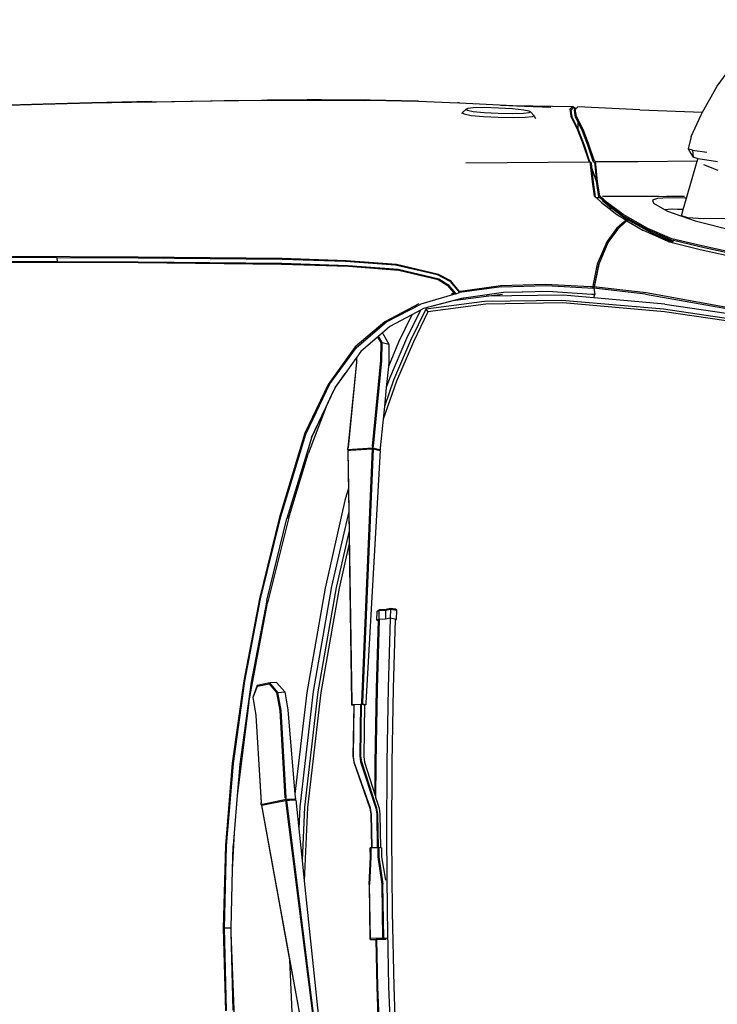
# Model space of a CAD drawing. Units: inches. Extents: x 22042254 to 25404563, y 17568978 to 17626777.
# Tile 13 of 45: x 22042340.9867 to 22042341.4576, y 17568978.1657 to 17568978.8305. Entities that reach past the tile are written whole.
import ezdxf

# ---------------------------------------------------------------- set-up
doc = ezdxf.new("R2010")
doc.units = ezdxf.units.IN
doc.header["$MEASUREMENT"] = 0
doc.layers.add('A-SITE-VEHI', color=8, linetype='Continuous', lineweight=18)
doc.layers.add('Edges', color=250, linetype='Continuous')

# ---------------------------------------------------------------- blocks, each defined once
blk = doc.blocks.new('Nissan Qashqai pl')
at = {"layer": 'Edges'}
for p, q in [((8.4387, 12.0674), (8.4359, 11.9861)), ((8.4397, 12.0674), (8.4369, 11.9861)), ((8.4517, 12.0674), (8.4489, 11.9858)), ((8.4541, 11.9857), (8.4568, 12.0669)), ((8.3575, 12.0475), (8.3104, 11.7881)), ((8.3406, 11.9567), (8.3448, 12.0536)), ((8.336, 11.7828), (8.3688, 12.0419)), ((8.3702, 12.0427), (8.3374, 11.7826)), ((8.3565, 11.8707), (8.3746, 12.0435)), ((8.2765, 11.9273), (8.2804, 12.0305)), ((8.2682, 11.9221), (8.2708, 12.0123)), ((8.2719, 12.0118), (8.2695, 11.9221)), ((8.2765, 11.9273), (8.2788, 12.0114)), ((8.3406, 11.9567), (8.3495, 12.0053)), ((8.4359, 11.9861), (8.4348, 11.9346)), ((8.4369, 11.9861), (8.4358, 11.9346)), ((8.4489, 11.9858), (8.4471, 11.9043)), ((8.4523, 11.9043), (8.4541, 11.9857)), ((8.31, 11.7882), (8.3406, 11.9567)), ((8.4272, 11.8746), (8.4281, 11.9336)), ((8.4287, 11.9335), (8.4278, 11.8745)), ((8.4281, 11.9336), (8.429, 11.9345)), ((8.4281, 11.9336), (8.4287, 11.9336)), ((8.4287, 11.9335), (8.4281, 11.9336)), ((8.429, 11.9345), (8.4287, 11.9336)), ((8.4287, 11.9336), (8.4287, 11.9335)), ((8.4418, 11.9332), (8.4287, 11.9335)), ((8.4328, 11.9347), (8.429, 11.9345)), ((8.429, 11.9345), (8.4326, 11.9345)), ((8.4328, 11.9347), (8.4326, 11.9345)), ((8.4326, 11.9345), (8.4348, 11.9344)), ((8.4348, 11.9346), (8.4328, 11.9347)), ((8.4348, 11.9346), (8.4348, 11.9344)), ((8.4358, 11.9346), (8.4348, 11.9346)), ((8.4348, 11.9344), (8.4358, 11.9344)), ((8.4358, 11.9346), (8.4358, 11.9344)), ((8.4459, 11.9344), (8.4358, 11.9346)), ((8.4358, 11.9344), (8.4422, 11.9342)), ((8.441, 11.8742), (8.4418, 11.9332)), ((8.4418, 11.9332), (8.4422, 11.9342)), ((8.4431, 11.9332), (8.4418, 11.9332)), ((8.4422, 11.9342), (8.4459, 11.9344)), ((8.4422, 11.9342), (8.4431, 11.9332)), ((8.4431, 11.9332), (8.4422, 11.8742)), ((8.4464, 11.9334), (8.4431, 11.9332)), ((8.4459, 11.9344), (8.4459, 11.9344)), ((8.2708, 11.8319), (8.2682, 11.9221)), ((8.2763, 11.9223), (8.2695, 11.9221)), ((8.2695, 11.9221), (8.2763, 11.9219)), ((8.2695, 11.9221), (8.2719, 11.8323)), ((8.2763, 11.9223), (8.2764, 11.9263)), ((8.2763, 11.9219), (8.2763, 11.9223)), ((8.2781, 11.8585), (8.2763, 11.9219)), ((8.2764, 11.9263), (8.2765, 11.9273)), ((8.4471, 11.9043), (8.4464, 11.8227)), ((8.4516, 11.823), (8.4523, 11.9043)), ((8.3542, 11.8485), (8.3565, 11.8707)), ((8.3599, 11.7906), (8.3565, 11.8707)), ((8.4272, 11.8746), (8.4286, 11.8445)), ((8.4292, 11.8445), (8.4278, 11.8745)), ((8.4368, 11.8443), (8.441, 11.8742)), ((8.438, 11.8443), (8.4422, 11.8742)), ((8.4408, 11.8444), (8.4452, 11.8698)), ((8.28, 11.818), (8.2781, 11.8585)), ((8.2788, 11.8327), (8.2781, 11.8585)), ((8.2789, 11.8319), (8.2781, 11.8585)), ((8.3505, 11.8139), (8.3542, 11.8485)), ((8.3567, 11.7903), (8.3542, 11.8485)), ((8.4286, 11.8445), (8.4285, 11.8345)), ((8.4291, 11.8345), (8.4292, 11.8445)), ((8.4366, 11.8345), (8.4368, 11.8443)), ((8.4379, 11.8345), (8.438, 11.8443)), ((8.4406, 11.8344), (8.4408, 11.8444)), ((8.2719, 11.8323), (8.2793, 11.7426)), ((8.2789, 11.8319), (8.2788, 11.8327)), ((8.4291, 11.8345), (8.4285, 11.8345)), ((8.4298, 11.8345), (8.4291, 11.8345)), ((8.4292, 11.7978), (8.4298, 11.8345)), ((8.4304, 11.8345), (8.4298, 11.7978)), ((8.4304, 11.8345), (8.4298, 11.8345)), ((8.436, 11.8344), (8.4304, 11.8345)), ((8.4355, 11.7977), (8.436, 11.8344)), ((8.4366, 11.8343), (8.436, 11.8344)), ((8.4366, 11.8345), (8.4379, 11.8345)), ((8.4366, 11.8344), (8.4366, 11.8345)), ((8.4373, 11.8344), (8.4366, 11.8344)), ((8.4373, 11.8344), (8.4366, 11.8343)), ((8.4366, 11.8343), (8.4366, 11.8344)), ((8.4373, 11.8344), (8.4367, 11.7977)), ((8.4379, 11.8344), (8.4373, 11.8344)), ((8.4379, 11.8343), (8.4373, 11.8344)), ((8.4379, 11.8344), (8.4379, 11.8345)), ((8.4397, 11.8344), (8.4379, 11.8343)), ((8.4379, 11.8343), (8.4379, 11.8344)), ((8.4391, 11.7978), (8.4397, 11.8344)), ((8.4406, 11.8344), (8.4397, 11.8344)), ((8.2781, 11.7423), (8.2708, 11.8319)), ((8.28, 11.818), (8.2789, 11.8319)), ((8.4464, 11.8227), (8.4468, 11.7413)), ((8.452, 11.7418), (8.4516, 11.823)), ((8.2834, 11.7773), (8.28, 11.818)), ((8.3472, 11.7821), (8.3505, 11.8139)), ((8.3516, 11.79), (8.3505, 11.8139)), ((8.3662, 11.6639), (8.3516, 11.79)), ((8.3713, 11.6645), (8.3567, 11.7903)), ((8.3745, 11.665), (8.3599, 11.7906)), ((8.4107, 11.7411), (8.4281, 11.7914)), ((8.4287, 11.7914), (8.4111, 11.741)), ((8.4179, 11.7406), (8.4344, 11.7912)), ((8.4357, 11.7912), (8.4193, 11.7407)), ((8.4281, 11.7914), (8.4292, 11.7978)), ((8.4298, 11.7978), (8.4287, 11.7914)), ((8.4344, 11.7912), (8.4355, 11.7977)), ((8.4347, 11.7805), (8.4381, 11.7914)), ((8.4367, 11.7977), (8.4357, 11.7912)), ((8.4381, 11.7914), (8.4391, 11.7978)), ((8.3038, 11.6903), (8.3095, 11.7853)), ((8.3099, 11.7851), (8.3042, 11.6901)), ((8.3092, 11.7863), (8.3093, 11.7873)), ((8.3092, 11.7863), (8.3099, 11.7851)), ((8.3095, 11.7853), (8.3092, 11.7863)), ((8.3093, 11.7873), (8.3367, 11.7816)), ((8.3159, 11.7869), (8.3093, 11.7873)), ((8.31, 11.7882), (8.3104, 11.7881)), ((8.3104, 11.7881), (8.3159, 11.7869)), ((8.3159, 11.7869), (8.336, 11.7828)), ((8.3298, 11.6848), (8.3355, 11.7798)), ((8.3369, 11.7796), (8.3312, 11.6846)), ((8.3355, 11.7798), (8.3366, 11.7806)), ((8.336, 11.7828), (8.3374, 11.7826)), ((8.3367, 11.7816), (8.3366, 11.7806)), ((8.3366, 11.7806), (8.3369, 11.7796)), ((8.3367, 11.7816), (8.347, 11.7811)), ((8.3374, 11.7826), (8.3406, 11.7824)), ((8.3458, 11.7813), (8.3406, 11.7824)), ((8.3406, 11.7824), (8.3457, 11.7821)), ((8.3458, 11.7813), (8.3457, 11.7821)), ((8.3457, 11.7821), (8.3472, 11.7821)), ((8.347, 11.7811), (8.3458, 11.7813)), ((8.3464, 11.7761), (8.3467, 11.7791)), ((8.3467, 11.7791), (8.347, 11.7811)), ((8.4337, 11.7775), (8.4347, 11.7805)), ((8.4347, 11.7805), (8.4348, 11.7421)), ((8.296, 11.6762), (8.2834, 11.7773)), ((8.2862, 11.7434), (8.2834, 11.7773)), ((8.3385, 11.6842), (8.3464, 11.7761)), ((8.3593, 11.6651), (8.3464, 11.7761)), ((8.4222, 11.7413), (8.4337, 11.7775)), ((8.4337, 11.7775), (8.4339, 11.7423)), ((8.2905, 11.6524), (8.2781, 11.7423)), ((8.2793, 11.7426), (8.2916, 11.6528)), ((8.2985, 11.654), (8.2862, 11.7434)), ((8.4097, 11.7348), (8.4107, 11.7411)), ((8.4111, 11.741), (8.41, 11.7346)), ((8.417, 11.7342), (8.4179, 11.7406)), ((8.4193, 11.7407), (8.4183, 11.7343)), ((8.4213, 11.735), (8.4222, 11.7413)), ((8.4339, 11.7423), (8.4353, 11.6613)), ((8.4348, 11.7421), (8.4362, 11.661)), ((8.4468, 11.7413), (8.4482, 11.66)), ((8.4534, 11.6608), (8.452, 11.7418)), ((8.4104, 11.6791), (8.4097, 11.7348)), ((8.41, 11.7346), (8.4108, 11.6791)), ((8.4177, 11.678), (8.417, 11.7342)), ((8.4183, 11.7343), (8.4191, 11.678)), ((8.4221, 11.6787), (8.4213, 11.735)), ((8.3005, 11.6706), (8.3038, 11.6903)), ((8.3042, 11.6901), (8.3009, 11.6704)), ((8.3264, 11.6652), (8.3298, 11.6848)), ((8.3312, 11.6846), (8.3278, 11.665)), ((8.3352, 11.6646), (8.3385, 11.6842)), ((8.296, 11.6762), (8.3166, 11.5675)), ((8.4086, 11.6764), (8.4045, 11.4011)), ((8.4056, 11.5028), (8.4082, 11.6766)), ((8.4082, 11.6785), (8.4104, 11.6791)), ((8.4082, 11.6785), (8.4086, 11.6784)), ((8.4082, 11.6766), (8.4082, 11.6785)), ((8.4086, 11.6784), (8.4086, 11.6764)), ((8.4086, 11.6784), (8.4117, 11.6782)), ((8.4104, 11.6791), (8.4108, 11.6791)), ((8.4104, 11.6786), (8.4104, 11.6791)), ((8.4108, 11.6786), (8.4104, 11.6786)), ((8.4104, 11.6786), (8.4108, 11.6784)), ((8.4108, 11.6791), (8.4108, 11.6786)), ((8.4108, 11.6786), (8.4108, 11.6784)), ((8.4108, 11.6784), (8.4117, 11.6783)), ((8.4117, 11.6783), (8.4117, 11.6782)), ((8.4117, 11.6783), (8.4177, 11.678)), ((8.4117, 11.6782), (8.419, 11.6778)), ((8.4177, 11.678), (8.4191, 11.678)), ((8.419, 11.6778), (8.4203, 11.6778)), ((8.419, 11.6758), (8.419, 11.6778)), ((8.4305, 11.3996), (8.419, 11.6758)), ((8.4191, 11.678), (8.4221, 11.6787)), ((8.4238, 11.6786), (8.4203, 11.6778)), ((8.4203, 11.6778), (8.4204, 11.6758)), ((8.4204, 11.6758), (8.4319, 11.3996)), ((8.4238, 11.6786), (8.4221, 11.6787)), ((8.4238, 11.6766), (8.4238, 11.6786)), ((8.4394, 11.4014), (8.4238, 11.6766)), ((8.3053, 11.6574), (8.3005, 11.6706)), ((8.3009, 11.6704), (8.3054, 11.6583)), ((8.3182, 11.6557), (8.3264, 11.6652)), ((8.3278, 11.665), (8.319, 11.6546)), ((8.3264, 11.6542), (8.3352, 11.6646)), ((8.3278, 11.665), (8.3352, 11.6646)), ((8.3792, 11.5515), (8.3593, 11.6651)), ((8.3864, 11.5497), (8.3662, 11.6639)), ((8.3913, 11.5506), (8.3713, 11.6645)), ((8.3945, 11.5513), (8.3745, 11.665)), ((8.4353, 11.6613), (8.4375, 11.5863)), ((8.4362, 11.661), (8.4385, 11.5858)), ((8.4557, 11.5855), (8.4534, 11.6608)), ((8.3076, 11.5631), (8.2905, 11.6524)), ((8.2916, 11.6528), (8.3089, 11.5631)), ((8.3157, 11.5647), (8.2985, 11.654)), ((8.3054, 11.6583), (8.3053, 11.6574)), ((8.319, 11.6546), (8.3053, 11.6574)), ((8.3054, 11.6583), (8.3182, 11.6557)), ((8.319, 11.6546), (8.3182, 11.6557)), ((8.3264, 11.6542), (8.319, 11.6546)), ((8.4482, 11.66), (8.4505, 11.5843)), ((8.4377, 11.5857), (8.4357, 11.5864)), ((8.4357, 11.5864), (8.4359, 11.5765)), ((8.4357, 11.5864), (8.4375, 11.5863)), ((8.4375, 11.5863), (8.4375, 11.5862)), ((8.4379, 11.5758), (8.4377, 11.5857)), ((8.445, 11.5853), (8.4377, 11.5857)), ((8.4452, 11.5754), (8.445, 11.5853)), ((8.4503, 11.5841), (8.445, 11.5853)), ((8.4572, 11.5854), (8.4503, 11.5841)), ((8.4557, 11.5855), (8.4572, 11.5854)), ((8.4557, 11.5853), (8.4557, 11.5855)), ((8.4572, 11.5854), (8.4574, 11.5755)), ((8.4359, 11.5765), (8.4379, 11.5758)), ((8.4359, 11.5765), (8.4377, 11.5753)), ((8.4387, 11.5749), (8.4377, 11.5753)), ((8.4379, 11.5758), (8.4452, 11.5754)), ((8.4384, 11.5752), (8.4457, 11.5749)), ((8.446, 11.5746), (8.4387, 11.5749)), ((8.4452, 11.5754), (8.4505, 11.5742)), ((8.4507, 11.5734), (8.446, 11.5746)), ((8.4505, 11.5742), (8.4503, 11.5841)), ((8.4505, 11.5742), (8.4574, 11.5755)), ((8.4574, 11.5755), (8.4559, 11.5744)), ((8.3157, 11.5647), (8.3377, 11.4753)), ((8.3392, 11.4758), (8.3166, 11.5675)), ((8.4507, 11.5734), (8.4505, 11.5742)), ((8.4559, 11.5744), (8.4507, 11.5734)), ((8.3296, 11.4739), (8.3076, 11.5631)), ((8.3089, 11.5631), (8.3311, 11.4733)), ((8.4009, 11.4559), (8.3792, 11.5515)), ((8.4051, 11.4678), (8.3864, 11.5497)), ((8.4054, 11.4887), (8.3913, 11.5506)), ((8.4056, 11.5028), (8.3945, 11.5513)), ((8.4054, 11.4887), (8.4056, 11.5028)), ((8.4051, 11.4678), (8.4054, 11.4887)), ((8.3573, 11.3824), (8.3296, 11.4739)), ((8.3311, 11.4733), (8.3582, 11.3836)), ((8.3648, 11.3863), (8.3377, 11.4753)), ((8.3392, 11.4758), (8.3608, 11.4048)), ((8.4048, 11.4423), (8.4051, 11.4678)), ((8.4048, 11.4423), (8.4009, 11.4559)), ((8.4041, 11.4013), (8.4048, 11.4423)), ((8.3799, 11.3545), (8.3608, 11.4048)), ((8.407, 11.401), (8.4037, 11.4002)), ((8.4037, 11.4002), (8.4314, 11.3985)), ((8.4037, 11.3992), (8.4037, 11.4002)), ((8.4037, 11.3992), (8.4046, 11.3981)), ((8.4042, 11.3983), (8.4037, 11.3992)), ((8.4041, 11.4013), (8.4045, 11.4011)), ((8.4134, 11.3049), (8.4042, 11.3983)), ((8.4045, 11.4011), (8.407, 11.401)), ((8.4046, 11.3981), (8.4138, 11.3048)), ((8.407, 11.401), (8.4305, 11.3996)), ((8.4305, 11.3996), (8.4319, 11.3996)), ((8.4306, 11.3966), (8.4314, 11.3975)), ((8.4398, 11.3032), (8.4306, 11.3966)), ((8.4314, 11.3985), (8.4394, 11.4004)), ((8.4314, 11.3985), (8.4314, 11.3975)), ((8.4314, 11.3975), (8.4319, 11.3967)), ((8.4319, 11.3996), (8.436, 11.4006)), ((8.4319, 11.3967), (8.4412, 11.3033)), ((8.436, 11.4006), (8.4394, 11.4014)), ((8.4394, 11.4004), (8.436, 11.4006)), ((8.4394, 11.3984), (8.4394, 11.4004)), ((8.4425, 11.3672), (8.4394, 11.3984)), ((8.3826, 11.3291), (8.3573, 11.3824)), ((8.3582, 11.3836), (8.3844, 11.3284)), ((8.3646, 11.387), (8.3799, 11.3545)), ((8.3888, 11.3355), (8.3648, 11.3863)), ((8.4571, 11.3258), (8.4425, 11.3672)), ((8.4439, 11.3531), (8.4425, 11.3672)), ((8.3799, 11.3545), (8.3888, 11.3355)), ((8.454, 11.3245), (8.4439, 11.3531)), ((8.4459, 11.3326), (8.4439, 11.3531)), ((8.4122, 11.2883), (8.3826, 11.3291)), ((8.3844, 11.3284), (8.4134, 11.2888)), ((8.3901, 11.3328), (8.3888, 11.3355)), ((8.3901, 11.3328), (8.4011, 11.3173)), ((8.3904, 11.3321), (8.3901, 11.3328)), ((8.4011, 11.3173), (8.3904, 11.3321)), ((8.4493, 11.3229), (8.4459, 11.3326)), ((8.4482, 11.3095), (8.4459, 11.3326)), ((8.4135, 11.3), (8.4011, 11.3173)), ((8.468, 11.2793), (8.4493, 11.3229)), ((8.4725, 11.2812), (8.454, 11.3245)), ((8.4756, 11.2826), (8.4571, 11.3258)), ((8.4594, 11.2831), (8.4482, 11.3095)), ((8.4487, 11.305), (8.4482, 11.3095)), ((8.4135, 11.3), (8.4134, 11.3049)), ((8.4139, 11.2994), (8.4135, 11.3)), ((8.4138, 11.3048), (8.4139, 11.2994)), ((8.4183, 11.2934), (8.4139, 11.2994)), ((8.44, 11.2834), (8.4398, 11.3032)), ((8.4412, 11.3033), (8.4415, 11.2835)), ((8.4489, 11.2852), (8.4487, 11.305)), ((8.4444, 11.2608), (8.4122, 11.2883)), ((8.4134, 11.2888), (8.4462, 11.2609)), ((8.4365, 11.2776), (8.4183, 11.2934)), ((8.4415, 11.2835), (8.4489, 11.2852)), ((8.4422, 11.2737), (8.4489, 11.2852)), ((8.4365, 11.2776), (8.44, 11.2834)), ((8.4375, 11.2767), (8.4365, 11.2776)), ((8.4415, 11.2835), (8.4375, 11.2767)), ((8.4412, 11.2735), (8.4375, 11.2767)), ((8.4737, 11.2534), (8.4594, 11.2831)), ((8.4831, 11.2484), (8.468, 11.2793)), ((8.4889, 11.2473), (8.4725, 11.2812)), ((8.4914, 11.25), (8.4756, 11.2826)), ((8.4422, 11.2737), (8.4412, 11.2735)), ((8.4499, 11.2659), (8.4412, 11.2735)), ((8.4737, 11.2534), (8.4499, 11.2659)), ((8.8745, 11.266), (8.7481, 11.2473)), ((8.8754, 11.2687), (8.7491, 11.2501)), ((8.4814, 11.2413), (8.4444, 11.2608)), ((8.4462, 11.2609), (8.4838, 11.2415)), ((8.4831, 11.2484), (8.4737, 11.2534)), ((8.7287, 11.2307), (8.8666, 11.2554)), ((8.8666, 11.2541), (8.7292, 11.2295)), ((8.7496, 11.2416), (8.8761, 11.2602)), ((8.4867, 11.2465), (8.4831, 11.2484)), ((8.528, 11.2354), (8.4867, 11.2465)), ((8.5214, 11.2374), (8.4867, 11.2465)), ((8.4889, 11.2473), (8.4914, 11.25)), ((8.5531, 11.2387), (8.4889, 11.2473)), ((8.5544, 11.2416), (8.4914, 11.25)), ((8.7481, 11.2473), (8.6375, 11.2376)), ((8.7491, 11.2501), (8.6386, 11.2404)), ((8.5216, 11.2303), (8.4838, 11.2415)), ((8.5214, 11.2374), (8.555, 11.233)), ((8.5301, 11.2352), (8.5214, 11.2374)), ((8.5736, 11.2291), (8.528, 11.2354)), ((8.6375, 11.2376), (8.5531, 11.2387)), ((8.6386, 11.2404), (8.5544, 11.2416)), ((8.6387, 11.2319), (8.555, 11.233)), ((8.555, 11.233), (8.5726, 11.2307)), ((8.6699, 11.231), (8.622, 11.228)), ((8.6721, 11.2348), (8.6387, 11.2319)), ((8.6721, 11.2312), (8.6699, 11.231)), ((8.7496, 11.2416), (8.6721, 11.2348)), ((8.6721, 11.2348), (8.6733, 11.2313)), ((8.6721, 11.2312), (8.6721, 11.2318)), ((8.6721, 11.2241), (8.6733, 11.2313)), ((8.6733, 11.2313), (8.6721, 11.2312)), ((8.5025, 11.2148), (8.5125, 11.221)), ((8.5125, 11.221), (8.5177, 11.2272)), ((8.5132, 11.2202), (8.5216, 11.2303)), ((8.5155, 11.2168), (8.5258, 11.2291)), ((8.5237, 11.2252), (8.5163, 11.2162)), ((8.5197, 11.2297), (8.5166, 11.2307)), ((8.5177, 11.2272), (8.5197, 11.2297)), ((8.5216, 11.2303), (8.5197, 11.2297)), ((8.5216, 11.2303), (8.5258, 11.2291)), ((8.5259, 11.2279), (8.5237, 11.2252)), ((8.5258, 11.2291), (8.5259, 11.2279)), ((8.5715, 11.2227), (8.5258, 11.2291)), ((8.5294, 11.2274), (8.5259, 11.2279)), ((8.5706, 11.2216), (8.5294, 11.2274)), ((8.6197, 11.2201), (8.5706, 11.2216)), ((8.5715, 11.2227), (8.6203, 11.2213)), ((8.5941, 11.2286), (8.5736, 11.2291)), ((8.5941, 11.2289), (8.5941, 11.2286)), ((8.622, 11.228), (8.5941, 11.2286)), ((8.6683, 11.2226), (8.6197, 11.2201)), ((8.6203, 11.2213), (8.6721, 11.2241)), ((8.671, 11.2227), (8.6683, 11.2226)), ((8.6721, 11.2241), (8.671, 11.2227)), ((8.6716, 11.2199), (8.671, 11.2227)), ((8.7287, 11.2307), (8.6721, 11.2241)), ((8.6721, 11.2241), (8.6727, 11.2229)), ((8.6772, 11.1988), (8.6721, 11.2241)), ((8.6753, 11.2232), (8.6727, 11.2229)), ((8.6777, 11.1984), (8.6727, 11.2229)), ((8.7292, 11.2295), (8.6753, 11.2232)), ((8.5018, 11.2098), (8.4559, 11.1991)), ((8.4588, 11.2036), (8.5032, 11.2141)), ((8.4595, 11.2047), (8.5025, 11.2148)), ((8.5155, 11.2168), (8.5018, 11.2098)), ((8.5163, 11.2162), (8.5029, 11.2092)), ((8.5032, 11.2141), (8.5132, 11.2202)), ((8.6759, 11.1982), (8.6716, 11.2199)), ((8.3318, 11.198), (8.4049, 11.2004)), ((8.332, 11.1971), (8.4042, 11.1995)), ((8.4559, 11.1991), (8.4014, 11.1953)), ((8.4042, 11.1995), (8.4588, 11.2036)), ((8.4049, 11.2004), (8.4595, 11.2047)), ((8.5029, 11.2092), (8.4571, 11.1983)), ((8.6875, 11.1744), (8.6772, 11.1988)), ((8.7881, 11.1821), (8.8918, 11.205)), ((8.8941, 11.2023), (8.7925, 11.1802)), ((8.8942, 11.2009), (8.7931, 11.1789)), ((8.0273, 11.1957), (8.1753, 11.1963)), ((8.0275, 11.1948), (8.0876, 11.1951)), ((8.0873, 11.1911), (8.0275, 11.1909)), ((8.1753, 11.1903), (8.0276, 11.1896)), ((8.0876, 11.1951), (8.0873, 11.1911)), ((8.1755, 11.1915), (8.0873, 11.1911)), ((8.0876, 11.1951), (8.1754, 11.1954)), ((8.1753, 11.1963), (8.3318, 11.198)), ((8.3324, 11.192), (8.1753, 11.1903)), ((8.1754, 11.1954), (8.332, 11.1971)), ((8.3324, 11.1931), (8.1755, 11.1915)), ((8.4014, 11.1953), (8.3324, 11.1931)), ((8.4022, 11.1943), (8.3324, 11.192)), ((8.4571, 11.1983), (8.4022, 11.1943)), ((8.6864, 11.1736), (8.6759, 11.1982)), ((8.6777, 11.1984), (8.6883, 11.1737)), ((8.7931, 11.1789), (8.7574, 11.1704)), ((8.7575, 11.1744), (8.7881, 11.1821)), ((8.7925, 11.1802), (8.7591, 11.1723)), ((8.697, 11.1592), (8.6864, 11.1736)), ((8.6979, 11.1603), (8.6875, 11.1744)), ((8.6883, 11.1737), (8.6987, 11.1597)), ((8.7508, 11.1722), (8.7257, 11.1609)), ((8.7529, 11.17), (8.7302, 11.1602)), ((8.7574, 11.1704), (8.7312, 11.1591)), ((8.7346, 11.1636), (8.7577, 11.1732)), ((8.7346, 11.1636), (8.7491, 11.1703)), ((8.7491, 11.1703), (8.7576, 11.1743)), ((8.7508, 11.1722), (8.7491, 11.1703)), ((8.7532, 11.1733), (8.7508, 11.1722)), ((8.7529, 11.17), (8.7577, 11.1732)), ((8.757, 11.1718), (8.7529, 11.17)), ((8.7532, 11.1733), (8.7575, 11.1744)), ((8.7587, 11.1722), (8.757, 11.1718)), ((8.7575, 11.1744), (8.7576, 11.1743)), ((8.7576, 11.1743), (8.7582, 11.1734)), ((8.7577, 11.1732), (8.7582, 11.1734)), ((8.7582, 11.1734), (8.759, 11.1725)), ((8.759, 11.1725), (8.7587, 11.1722)), ((8.7591, 11.1723), (8.7587, 11.1722)), ((8.759, 11.1725), (8.7591, 11.1723)), ((8.7055, 11.1514), (8.697, 11.1592)), ((8.6987, 11.1596), (8.6979, 11.1603)), ((8.6987, 11.1597), (8.6988, 11.1596)), ((8.6987, 11.1596), (8.6988, 11.1596)), ((8.6996, 11.1588), (8.6987, 11.1596)), ((8.6988, 11.1596), (8.6996, 11.1588)), ((8.6996, 11.1588), (8.6996, 11.1588)), ((8.7062, 11.1527), (8.6996, 11.1588)), ((8.6996, 11.1588), (8.7062, 11.1527)), ((8.7302, 11.1602), (8.7032, 11.145)), ((8.7312, 11.1591), (8.7042, 11.144)), ((8.7075, 11.1487), (8.7346, 11.1636)), ((8.7108, 11.1523), (8.7257, 11.1609)), ((8.7108, 11.1523), (8.7248, 11.1605)), ((8.7248, 11.1605), (8.7257, 11.1609)), ((8.7828, 11.1508), (8.8245, 11.1613)), ((8.6917, 11.1371), (8.7075, 11.1487)), ((8.7071, 11.15), (8.6981, 11.1446)), ((8.707, 11.15), (8.7055, 11.1514)), ((8.7067, 11.1522), (8.7062, 11.1527)), ((8.7083, 11.1508), (8.7067, 11.1522)), ((8.707, 11.15), (8.7083, 11.1508)), ((8.7071, 11.15), (8.707, 11.15)), ((8.707, 11.15), (8.707, 11.15)), ((8.7083, 11.1508), (8.7071, 11.15)), ((8.7083, 11.1507), (8.7102, 11.1519)), ((8.7083, 11.1508), (8.7083, 11.1507)), ((8.7102, 11.1519), (8.7108, 11.1523)), ((8.7524, 11.1401), (8.7828, 11.1508)), ((8.7748, 11.1475), (8.7678, 11.1453)), ((8.7678, 11.1453), (8.7698, 11.1385)), ((8.7916, 11.1488), (8.7748, 11.1475)), ((8.8259, 11.1483), (8.7916, 11.1488)), ((8.6805, 11.1309), (8.6884, 11.1371)), ((8.6818, 11.1288), (8.6902, 11.136)), ((8.6927, 11.1371), (8.6859, 11.132)), ((8.7042, 11.144), (8.687, 11.131)), ((8.6884, 11.1371), (8.6973, 11.144)), ((8.6884, 11.1371), (8.6917, 11.1371)), ((8.6902, 11.136), (8.6917, 11.1371)), ((8.6923, 11.1371), (8.6927, 11.1371)), ((8.7032, 11.145), (8.6927, 11.1371)), ((8.6973, 11.144), (8.698, 11.1446)), ((8.698, 11.1446), (8.6981, 11.1446)), ((8.7373, 11.1314), (8.7492, 11.1383)), ((8.7492, 11.1383), (8.7524, 11.1401)), ((8.7492, 11.1383), (8.7572, 11.1379)), ((8.7572, 11.1379), (8.7698, 11.1383)), ((8.7698, 11.1385), (8.7583, 11.1382)), ((8.7698, 11.1385), (8.7698, 11.1383)), ((8.7698, 11.1383), (8.7733, 11.126)), ((8.6714, 11.1088), (8.6737, 11.1245)), ((8.6727, 11.1235), (8.6737, 11.1245)), ((8.6737, 11.1245), (8.6746, 11.1253)), ((8.6805, 11.1309), (8.6746, 11.1253)), ((8.6746, 11.1253), (8.6785, 11.1253)), ((8.6777, 11.1246), (8.6755, 11.1099)), ((8.6788, 11.1237), (8.6764, 11.1083)), ((8.6785, 11.1253), (8.6777, 11.1246)), ((8.6815, 11.128), (8.6785, 11.1253)), ((8.687, 11.131), (8.6788, 11.1237)), ((8.6815, 11.128), (8.6818, 11.1288)), ((8.6817, 11.1282), (8.6815, 11.128)), ((8.6859, 11.132), (8.6817, 11.1282)), ((8.6817, 11.1282), (8.6818, 11.1288)), ((8.6818, 11.1238), (8.7026, 11.1238)), ((8.7026, 11.1238), (8.7026, 11.1239)), ((8.7026, 11.1238), (8.7072, 11.1239)), ((8.7072, 11.1239), (8.7072, 11.1239)), ((8.7072, 11.1239), (8.7273, 11.1239)), ((8.7273, 11.1239), (8.7273, 11.124)), ((8.7273, 11.1239), (8.7354, 11.124)), ((8.7354, 11.1241), (8.7354, 11.124)), ((8.7354, 11.124), (8.742, 11.124)), ((8.7361, 11.1283), (8.7373, 11.1314)), ((8.7415, 11.1265), (8.7361, 11.1283)), ((8.7534, 11.1257), (8.7415, 11.1265)), ((8.742, 11.1241), (8.742, 11.124)), ((8.742, 11.124), (8.742, 11.1241)), ((8.742, 11.124), (8.742, 11.124)), ((8.742, 11.124), (8.7426, 11.124)), ((8.7426, 11.1241), (8.7426, 11.124)), ((8.7426, 11.124), (8.7433, 11.124)), ((8.7433, 11.1241), (8.7433, 11.124)), ((8.7433, 11.124), (8.7711, 11.1241)), ((8.7711, 11.1241), (8.7516, 11.1241)), ((8.7718, 11.126), (8.7534, 11.1257)), ((8.7733, 11.126), (8.7718, 11.126)), ((8.7733, 11.126), (8.7849, 11.0859)), ((8.6703, 11.1081), (8.6727, 11.1235)), ((8.6684, 11.0892), (8.6703, 11.1081)), ((8.6697, 11.0922), (8.6714, 11.1088)), ((8.6698, 11.0925), (8.6755, 11.1099)), ((8.6754, 11.1089), (8.6735, 11.0898)), ((8.6764, 11.1082), (8.6744, 11.0891)), ((8.6755, 11.1099), (8.6754, 11.1089)), ((8.6764, 11.1082), (8.6764, 11.1083)), ((8.6692, 11.0876), (8.6697, 11.0922)), ((8.6697, 11.0922), (8.6698, 11.0925)), ((8.7917, 11.0895), (8.8075, 11.0955)), ((8.5326, 11.0874), (8.6675, 11.0866)), ((8.6606, 11.0674), (8.6667, 11.0857)), ((8.6616, 11.0683), (8.6675, 11.0862)), ((8.6718, 11.0868), (8.6657, 11.0684)), ((8.6667, 11.0857), (8.6675, 11.0862)), ((8.6728, 11.0858), (8.6667, 11.0675)), ((8.6674, 11.0864), (8.6675, 11.0865)), ((8.6675, 11.0865), (8.6675, 11.0866)), ((8.6676, 11.0866), (8.6675, 11.0866)), ((8.6675, 11.0862), (8.6679, 11.0864)), ((8.6676, 11.0864), (8.6677, 11.0866)), ((8.6677, 11.0866), (8.6676, 11.0866)), ((8.6682, 11.0866), (8.6677, 11.0866)), ((8.6679, 11.0864), (8.6682, 11.0866)), ((8.6682, 11.087), (8.6684, 11.0888)), ((8.6692, 11.0876), (8.6682, 11.0866)), ((8.6682, 11.087), (8.6692, 11.0876)), ((8.6682, 11.0866), (8.6682, 11.087)), ((8.6684, 11.0888), (8.6684, 11.0892)), ((8.6684, 11.0888), (8.6685, 11.089)), ((8.6729, 11.0874), (8.6718, 11.0868)), ((8.674, 11.0864), (8.6728, 11.0858)), ((8.6733, 11.0875), (8.6729, 11.0874)), ((8.6735, 11.0898), (8.6733, 11.0875)), ((8.6742, 11.0866), (8.674, 11.0864)), ((8.6744, 11.0891), (8.6742, 11.0866)), ((8.6744, 11.0866), (8.6742, 11.0866)), ((8.6742, 11.0858), (8.6743, 11.086)), ((8.6744, 11.0864), (8.6744, 11.0866)), ((8.6773, 11.0865), (8.6744, 11.0866)), ((8.6791, 11.0864), (8.677, 11.0864)), ((8.6791, 11.0865), (8.6773, 11.0865)), ((8.6791, 11.0865), (8.6791, 11.0864)), ((8.6878, 11.0864), (8.6791, 11.0865)), ((8.7205, 11.0863), (8.6791, 11.0864)), ((8.6878, 11.0864), (8.6791, 11.0864)), ((8.6878, 11.0865), (8.6878, 11.0864)), ((8.6911, 11.0864), (8.6878, 11.0864)), ((8.7205, 11.0863), (8.6911, 11.0864)), ((8.7849, 11.0859), (8.7205, 11.0863)), ((8.7779, 11.0773), (8.7807, 11.0812)), ((8.7798, 11.0739), (8.7807, 11.0812)), ((8.7849, 11.0827), (8.7807, 11.0812)), ((8.7849, 11.0859), (8.7856, 11.0834)), ((8.7849, 11.0827), (8.7858, 11.0828)), ((8.7858, 11.0828), (8.7856, 11.0834)), ((8.7858, 11.0828), (8.807, 11.0862)), ((8.7751, 11.0723), (8.7779, 11.0773)), ((8.7798, 11.0739), (8.7751, 11.0723)), ((8.7785, 11.0587), (8.7751, 11.0723)), ((8.7798, 11.0739), (8.7954, 11.0758)), ((8.6546, 11.0516), (8.6606, 11.0674)), ((8.6556, 11.0524), (8.6616, 11.0683)), ((8.6657, 11.0684), (8.6598, 11.0529)), ((8.6667, 11.0675), (8.6608, 11.0521)), ((8.6472, 11.0366), (8.6546, 11.0516)), ((8.6482, 11.0375), (8.655, 11.0513)), ((8.6608, 11.0521), (8.6534, 11.0369)), ((8.6598, 11.0529), (8.655, 11.0432)), ((8.655, 11.0513), (8.6556, 11.0524)), ((8.655, 11.0513), (8.655, 11.0432)), ((8.7785, 11.0587), (8.7891, 11.0353)), ((8.568, 11.0382), (8.5518, 11.0375)), ((8.5842, 11.0384), (8.568, 11.0382)), ((8.5974, 11.0381), (8.5842, 11.0384)), ((8.6049, 11.0373), (8.5974, 11.0381)), ((8.609, 11.0397), (8.6073, 11.0362)), ((8.6524, 11.0378), (8.651, 11.0302)), ((8.655, 11.0432), (8.6524, 11.0378)), ((8.5283, 11.0336), (8.5287, 11.0329)), ((8.531, 11.0346), (8.5287, 11.0329)), ((8.5287, 11.0329), (8.5331, 11.0292)), ((8.5385, 11.0363), (8.531, 11.0346)), ((8.5331, 11.0292), (8.5346, 11.0303)), ((8.5347, 11.0282), (8.5331, 11.0292)), ((8.5346, 11.0303), (8.5406, 11.0316)), ((8.5407, 11.0274), (8.5347, 11.0282)), ((8.5518, 11.0375), (8.5385, 11.0363)), ((8.5406, 11.0316), (8.5526, 11.0328)), ((8.5527, 11.0273), (8.5407, 11.0274)), ((8.5526, 11.0328), (8.5681, 11.0335)), ((8.5682, 11.0278), (8.5527, 11.0273)), ((8.5681, 11.0335), (8.5836, 11.0337)), ((8.5837, 11.0288), (8.5682, 11.0278)), ((8.5836, 11.0337), (8.5957, 11.0334)), ((8.5958, 11.0301), (8.5837, 11.0288)), ((8.5957, 11.0334), (8.6017, 11.0328)), ((8.6018, 11.0312), (8.5958, 11.0301)), ((8.6017, 11.0328), (8.6032, 11.0321)), ((8.6032, 11.0321), (8.6018, 11.0312)), ((8.6073, 11.0362), (8.6032, 11.0321)), ((8.6073, 11.0362), (8.6049, 11.0373)), ((8.646, 11.0289), (8.6468, 11.0337)), ((8.6489, 11.0263), (8.646, 11.0289)), ((8.6468, 11.0337), (8.6472, 11.0366)), ((8.647, 11.03), (8.6468, 11.0337)), ((8.647, 11.03), (8.6482, 11.0375)), ((8.6498, 11.0273), (8.647, 11.03)), ((8.6527, 11.0286), (8.6489, 11.0263)), ((8.6524, 11.0289), (8.6498, 11.0273)), ((8.651, 11.0302), (8.652, 11.0292)), ((8.6534, 11.0369), (8.652, 11.0292)), ((8.652, 11.0292), (8.6524, 11.0289)), ((8.6524, 11.0289), (8.6527, 11.0286)), ((8.6527, 11.0286), (8.6537, 11.0275)), ((8.6547, 11.0265), (8.6537, 11.0275)), ((8.6537, 11.0275), (8.6537, 11.0275)), ((8.7222, 11.0298), (8.6547, 11.0265)), ((8.7222, 11.0298), (8.7908, 11.0322)), ((8.7891, 11.0353), (8.7908, 11.0322)), ((8.7908, 11.0322), (8.8066, 11.0041)), ((8.016, 11.0253), (8.0713, 11.0237)), ((8.0718, 11.0235), (8.0168, 11.0251)), ((8.0713, 11.0237), (8.1249, 11.0223)), ((8.1251, 11.0222), (8.0718, 11.0235)), ((8.1249, 11.0223), (8.1901, 11.021)), ((8.1902, 11.0208), (8.1251, 11.0222)), ((8.1901, 11.021), (8.1938, 11.021)), ((8.1902, 11.021), (8.1938, 11.021)), ((8.1904, 11.0209), (8.1902, 11.0208)), ((8.1904, 11.0209), (8.2543, 11.0198)), ((8.1938, 11.021), (8.1954, 11.0209)), ((8.1954, 11.0209), (8.2544, 11.02)), ((8.2544, 11.0198), (8.2543, 11.0199)), ((8.2543, 11.0198), (8.2544, 11.0198)), ((8.2544, 11.02), (8.3166, 11.0193)), ((8.2544, 11.0198), (8.2556, 11.0198)), ((8.2556, 11.0198), (8.256, 11.0198)), ((8.256, 11.0198), (8.2561, 11.0198)), ((8.2561, 11.0198), (8.2693, 11.0197)), ((8.2693, 11.0197), (8.2694, 11.0197)), ((8.2694, 11.0197), (8.3098, 11.0192)), ((8.3098, 11.0192), (8.3163, 11.0192)), ((8.3663, 11.019), (8.3163, 11.0192)), ((8.3597, 11.019), (8.3163, 11.0192)), ((8.3166, 11.0193), (8.3764, 11.0191)), ((8.3602, 11.019), (8.3597, 11.019)), ((8.3608, 11.019), (8.3602, 11.019)), ((8.3663, 11.019), (8.3608, 11.019)), ((8.3663, 11.019), (8.3764, 11.0191)), ((8.3757, 11.019), (8.3663, 11.019)), ((8.4282, 11.0193), (8.3757, 11.019)), ((8.3764, 11.0191), (8.4069, 11.0192)), ((8.4069, 11.0192), (8.4219, 11.0196)), ((8.4069, 11.0192), (8.4292, 11.0193)), ((8.4799, 11.0202), (8.4282, 11.0193)), ((8.4292, 11.0193), (8.4799, 11.0202)), ((8.4811, 11.0203), (8.4799, 11.0202)), ((8.4811, 11.0203), (8.5241, 11.022)), ((8.5259, 11.0221), (8.5241, 11.022)), ((8.5259, 11.0221), (8.5838, 11.0251)), ((8.5707, 11.0248), (8.5965, 11.0258)), ((8.5838, 11.0251), (8.6489, 11.0263)), ((8.5838, 11.0251), (8.5965, 11.0258)), ((8.5965, 11.0258), (8.6252, 11.0268)), ((8.8066, 11.0041), (8.8591, 10.9315))]:
    blk.add_line(p, q, dxfattribs=at)
blk = doc.blocks.new('CAR')
blk.add_blockref('Nissan Qashqai pl', (-9.7433, -11.9151))

msp = doc.modelspace()

# ---------------------------------------------------------------- block references
at = {"layer": 'A-SITE-VEHI', "xscale": -0.6191396643141144, "yscale": 0.6191396643141144, "zscale": 0.6191396643141144, "rotation": 180}
msp.add_blockref('CAR', (22042342.03736, 17568978.22147), dxfattribs=at)

doc.saveas('drawing.dxf')
